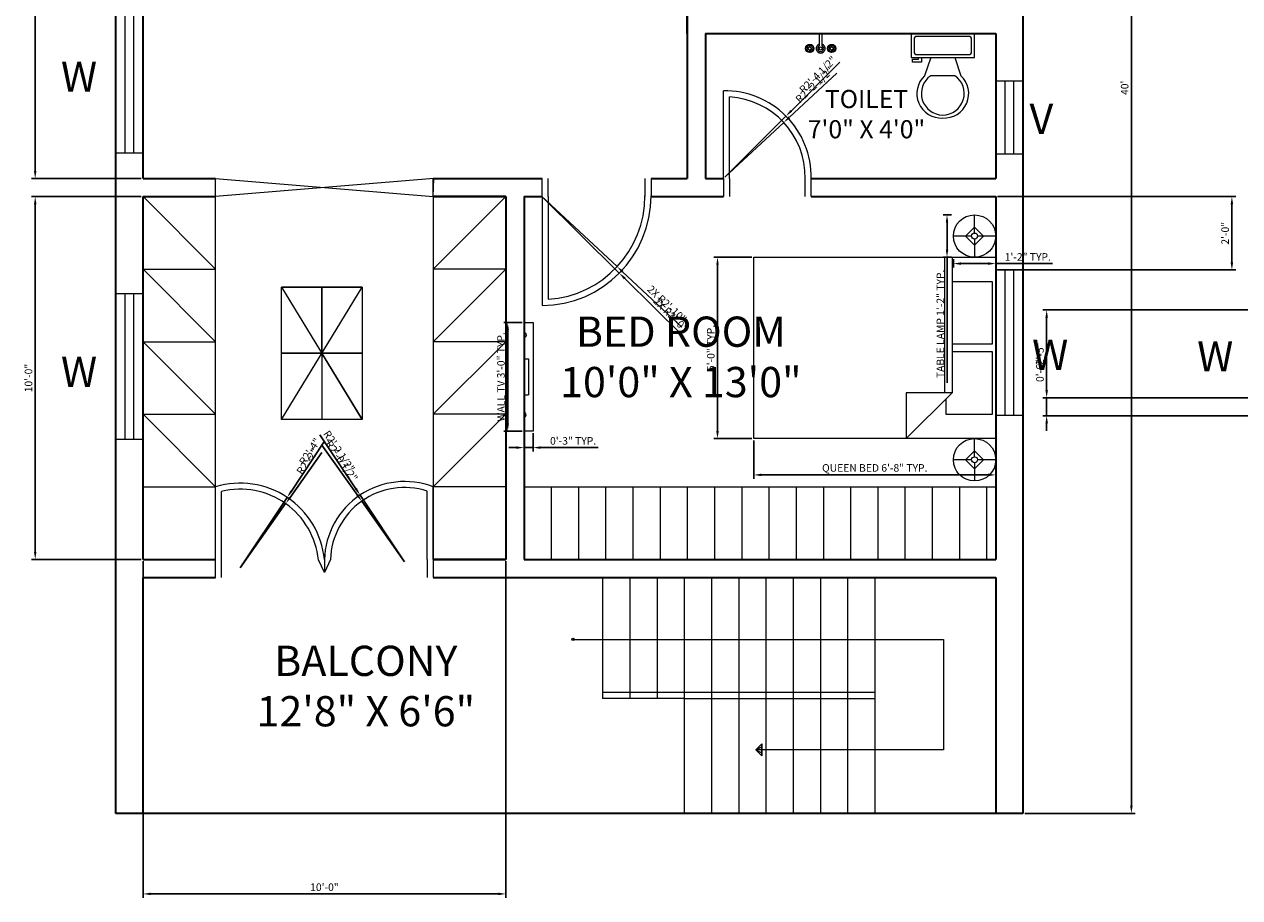
# Model space of a CAD drawing. Units: inches. Extents: x 2318 to 3542, y 1525 to 2117.
# Tile 3 of 6: x 2767 to 3169, y 1527 to 1816. Entities that reach past the tile are written whole.
import ezdxf

# ---------------------------------------------------------------- set-up
doc = ezdxf.new("R2010")
doc.units = ezdxf.units.IN
for name, color, linetype, lineweight in [('A-ANNO-DIMS', 2, 'Continuous', 18), ('A-ANNO-SYMB', 2, 'Continuous', 13), ('A-ANNO-TEXT', 7, 'Continuous', 18), ('A-AREA-IDEN', 7, 'Continuous', 25), ('A-DOOR', 4, 'Continuous', 18), ('A-EQPM', 9, 'Continuous', 18), ('A-FLOR-CASE', 8, 'Continuous', 18), ('A-FLOR-FIXT', 9, 'Continuous', 18), ('A-FLOR-STRS', 3, 'Continuous', 18), ('A-FURN', 8, 'Continuous', 18), ('A-GLAZ', 4, 'Continuous', 18), ('A-WALL', 7, 'Continuous', 35)]:
    doc.layers.add(name, color=color, linetype=linetype, lineweight=lineweight)
doc.styles.add('Annotative', font='arial.ttf')
doc.styles.get("Standard").update_dxf_attribs({"font": 'arial.ttf'})
doc.dimstyles.new('ISO-25', dxfattribs={"dimtxt": 2.5, "dimasz": 2.5, "dimexe": 1.25, "dimexo": 0.625, "dimtad": 1, "dimdec": 0, "dimlunit": 3, "dimtxsty": 'Standard', "dimcen": 2.5, "dimadec": 0, "dimazin": 0, "dimtfac": 1, "dimtdec": 0, "dimtmove": 0, "dimatfit": 3, "dimfxl": 1, "dimarcsym": 0})

# ---------------------------------------------------------------- blocks, each defined once
blk = doc.blocks.new('*D18')
at = {"layer": 'A-ANNO-DIMS', "color": 0, "lineweight": -2, "transparency": 16777216}
for p, q in [((3098.03, 2034.59), (3134.53, 2034.59)), ((3133.28, 2032.09), (3133.28, 1557.09)), ((3098.03, 1554.59), (3134.53, 1554.59))]:
    blk.add_line(p, q, dxfattribs=at)
at = {"layer": 'A-ANNO-DIMS', "color": 0, "transparency": 16777216}
for points in [[(3132.86, 2032.09), (3133.69, 2032.09), (3133.28, 2034.59)], [(3132.86, 1557.09), (3133.69, 1557.09), (3133.28, 1554.59)]]:
    blk.add_solid(points, dxfattribs=at)
at = {"layer": 'Defpoints', "color": 0, "transparency": 16777216}
for p in [(3097.41, 2034.59), (3097.41, 1554.59), (3133.28, 1554.59)]:
    blk.add_point(p, dxfattribs=at)
at = {"layer": 'A-ANNO-DIMS', "color": 0, "transparency": 16777216, "insert": (3131.38, 1794.59), "char_height": 2.5, "attachment_point": 5, "rotation": 90}
blk.add_mtext("40'", dxfattribs=at)
blk = doc.blocks.new('Bed - Queen')
for p, q in [((0, -80.00003), (0, 0)), ((0, 0), (59.99999, 0)), ((59.99999, 0), (59.99999, -80.00003)), ((7.99999, -1.2), (28.79998, -1.2)), ((7.99999, -14.4), (7.99999, -1.2)), ((28.79998, -1.2), (28.79998, -14.4)), ((31.19999, -1.2), (51.99999, -1.2)), ((31.19999, -14.4), (31.19999, -1.2)), ((51.99999, -1.2), (51.99999, -16.4)), ((0, -14.4), (44.8, -14.4)), ((59.99999, -29.6), (44.8, -14.4)), ((44.8, -14.4), (44.8, -29.6)), ((44.8, -16.8), (0, -16.8)), ((51.99999, -16.4), (46.79936, -16.4)), ((44.8, -29.6), (59.99999, -29.6)), ((59.99999, -80.00003), (0, -80.00003))]:
    blk.add_line(p, q)
blk = doc.blocks.new('Lamp - Table')
for p, q in [((0, 7), (0, 1)), ((-1, 0), (-7, 0)), ((0, 3), (-3, 0)), ((-3, 0), (0, -3)), ((3, 0), (0, 3)), ((0, -3), (3, 0)), ((1, 0), (7, 0)), ((0, -1), (0, -7))]:
    blk.add_line(p, q)
for radius in [7, 1]:
    blk.add_circle((0, 0), radius)
blk = doc.blocks.new('*U14')
for p, q in [((241.3, -152.4), (241.3, -50.8)), ((-203.2, -215.9), (-203.2, -203.2)), ((-177.8, -203.2), (-177.8, -241.3)), ((-101.6, -203.2), (-152.4, -355.6)), ((101.6, -203.2), (152.4, -355.6)), ((-254, -215.9), (-203.2, -215.9)), ((-254, -241.3), (-254, -215.9)), ((-177.8, -241.3), (-254, -241.3)), ((101.6, -355.6), (-101.6, -355.6))]:
    blk.add_line(p, q)
blk.add_lwpolyline([(266.7, -203.2), (266.7, 0), (-266.7, 0), (-266.7, -203.2)], close=True)
for points in [[(-241.3, -50.8), (-241.3, -152.4)], [(215.9, -25.4), (-215.9, -25.4)], [(-215.9, -177.8), (215.9, -177.8)]]:
    blk.add_lwpolyline(points)
for centre, radius, start, end in [((-219.075, -47.625), 22.45064, 81.8699, 188.1301), ((219.075, -47.625), 22.45064, 351.8699, 98.1301), ((-219.075, -155.575), 22.45064, 171.869898, 278.1301), ((219.075, -155.575), 22.45064, 261.8699, 8.1301), ((-12.12088, -505.93752), 205.61935, 133.01722, 273.38), ((0.94996, -504.77674), 181.02486, 124.50543, 269.7), ((-0.94742, -504.77674), 181.02486, 270.3, 55.4946), ((12.12342, -505.93752), 205.61935, 266.62, 46.9828)]:
    blk.add_arc(centre, radius, start, end)
blk = doc.blocks.new('Faucet - Bathroom top')
for p, q in [((-4.107, 0.125), (-4.375, 0.125)), ((-3.75, 0.4788), (-3.75, 0.75)), ((-3.5, 0.482), (-3.5, 0.75)), ((-3.1461, 0.125), (-2.875, 0.125)), ((3.143, 0.125), (2.875, 0.125)), ((3.5, 0.4788), (3.5, 0.75)), ((3.75, 0.482), (3.75, 0.75)), ((4.1039, 0.125), (4.375, 0.125)), ((-4.1039, -0.125), (-4.375, -0.125)), ((-3.75, -0.4821), (-3.75, -0.75)), ((-3.5, -0.4789), (-3.5, -0.75)), ((-3.143, -0.125), (-2.875, -0.125)), ((-0.5, -0.8639), (-0.5, -4.5)), ((0.5, -4.5), (0.5, -0.8631)), ((3.1461, -0.125), (2.875, -0.125)), ((3.5, -0.4821), (3.5, -0.75)), ((3.75, -0.4789), (3.75, -0.75)), ((4.107, -0.125), (4.375, -0.125))]:
    blk.add_line(p, q)
for centre, radius in [((-3.625, 0), 1.375), ((-4.625, 0), 0.2795), ((-3.625, 0), 0.5), ((-3.625, 1), 0.2795), ((-2.625, 0), 0.2795), ((0, 0), 0.5), ((3.625, 0), 1.375), ((2.625, 0), 0.2795), ((3.625, 0), 0.5), ((3.625, 1), 0.2795), ((4.625, 0), 0.2795), ((-3.625, -1), 0.2795), ((3.625, -1), 0.2795)]:
    blk.add_circle(centre, radius)
for centre, radius, start, end in [((-3.625, 0), 1, 105.2407, 164.2093), ((-3.625, 0), 1, 16.44125, 74.07887), ((0, 0), 1.5, 289.6514, 250.3603), ((0, 0), 1, 300.3431, 239.7554), ((3.625, 0), 1, 106.12, 164.0884), ((3.625, 0), 1, 16.23422, 73.90469), ((-3.625, 0), 1, 196.2342, 253.9047), ((-3.625, 0), 1, 286.12, 344.0884), ((3.625, 0), 1, 196.4413, 254.0789), ((3.625, 0), 1, 285.2407, 344.2093), ((0, -4.5), 0.5, 180, 0)]:
    blk.add_arc(centre, radius, start, end)
blk = doc.blocks.new('WIN-48x9')
for p, q in [((48, 9), (0, 9)), ((0, 9), (0, 0)), ((48, 0), (48, 9)), ((48, 6), (0, 6)), ((0, 3), (48, 3)), ((0, 0), (48, 0))]:
    blk.add_line(p, q)
blk = doc.blocks.new('VENT-24x9')
for p, q in [((0, 24), (0, 0)), ((9, 24), (0, 24)), ((3, 24), (3, 0)), ((6, 0), (6, 24)), ((9, 0), (9, 24)), ((0, 0), (9, 0))]:
    blk.add_line(p, q)
blk = doc.blocks.new('TV-36-WALL')
for p, q in [((0, 0), (0, 3)), ((0, 3), (36, 3)), ((0, 0), (0, 0)), ((0, 0), (24, 0)), ((0, 0), (12, 0)), ((12, 0), (12, 1.44)), ((12, 1.44), (23.97, 1.44)), ((23.97, 1.44), (24, 0)), ((24, 0), (23.97, 1.44)), ((36, 0), (24, 0)), ((36, 3), (36, 0))]:
    blk.add_line(p, q)
for centre, radius in [((4.16, 0), 0.848), ((30.54, 0), 0.733)]:
    blk.add_arc(centre, radius, 360, 180)
blk = doc.blocks.new('*D30')
at = {"layer": 'A-ANNO-DIMS', "color": 0, "lineweight": -2, "transparency": 16777216}
for p, q in [((3073.78, 1752.54), (3071.06, 1752.54)), ((3072.31, 1750.04), (3072.31, 1741.04)), ((3073.78, 1738.54), (3071.06, 1738.54)), ((3072.31, 1738.54), (3072.31, 1696.97))]:
    blk.add_line(p, q, dxfattribs=at)
at = {"layer": 'A-ANNO-DIMS', "color": 0, "transparency": 16777216}
for points in [[(3071.89, 1750.04), (3072.72, 1750.04), (3072.31, 1752.54)], [(3071.89, 1741.04), (3072.72, 1741.04), (3072.31, 1738.54)]]:
    blk.add_solid(points, dxfattribs=at)
at = {"layer": 'Defpoints', "color": 0, "transparency": 16777216}
for p in [(3074.41, 1752.54), (3072.31, 1738.54), (3074.41, 1738.54)]:
    blk.add_point(p, dxfattribs=at)
at = {"layer": 'A-ANNO-DIMS', "color": 0, "transparency": 16777216, "insert": (3070.43, 1716.5), "char_height": 2.5, "attachment_point": 5, "rotation": 90}
blk.add_mtext('TABLE LAMP 1\'-2" TYP.', dxfattribs=at)
blk = doc.blocks.new('*D31')
at = {"layer": 'A-ANNO-DIMS', "color": 0, "lineweight": -2, "transparency": 16777216}
for p, q in [((3074.41, 1737.91), (3074.41, 1735.19)), ((3076.91, 1736.44), (3085.91, 1736.44)), ((3088.41, 1737.91), (3088.41, 1735.19)), ((3088.41, 1736.44), (3107.16, 1736.44))]:
    blk.add_line(p, q, dxfattribs=at)
at = {"layer": 'A-ANNO-DIMS', "color": 0, "transparency": 16777216}
for points in [[(3076.91, 1736.86), (3076.91, 1736.02), (3074.41, 1736.44)], [(3085.91, 1736.86), (3085.91, 1736.02), (3088.41, 1736.44)]]:
    blk.add_solid(points, dxfattribs=at)
at = {"layer": 'Defpoints', "color": 0, "transparency": 16777216}
for p in [(3074.41, 1738.54), (3088.41, 1738.54), (3088.41, 1736.44)]:
    blk.add_point(p, dxfattribs=at)
at = {"layer": 'A-ANNO-DIMS', "color": 0, "transparency": 16777216, "insert": (3099.03, 1738.32), "char_height": 2.5, "attachment_point": 5}
blk.add_mtext('1\'-2" TYP.', dxfattribs=at)
blk = doc.blocks.new('*D36')
at = {"layer": 'A-ANNO-DIMS', "color": 0, "lineweight": -2, "transparency": 16777216}
for p, q in [((3008.41, 1677.91), (3008.41, 1665.29)), ((3088.41, 1677.91), (3088.41, 1665.29)), ((3010.91, 1666.54), (3085.91, 1666.54))]:
    blk.add_line(p, q, dxfattribs=at)
at = {"layer": 'A-ANNO-DIMS', "color": 0, "transparency": 16777216}
for points in [[(3010.91, 1666.96), (3010.91, 1666.12), (3008.41, 1666.54)], [(3085.91, 1666.96), (3085.91, 1666.12), (3088.41, 1666.54)]]:
    blk.add_solid(points, dxfattribs=at)
at = {"layer": 'Defpoints', "color": 0, "transparency": 16777216}
for p in [(3008.41, 1678.54), (3088.41, 1678.54), (3088.41, 1666.54)]:
    blk.add_point(p, dxfattribs=at)
at = {"layer": 'A-ANNO-DIMS', "color": 0, "transparency": 16777216, "insert": (3048.41, 1668.53), "char_height": 2.5, "attachment_point": 5}
blk.add_mtext('QUEEN BED 6\'-8" TYP.', dxfattribs=at)
blk = doc.blocks.new('*D37')
at = {"layer": 'A-ANNO-DIMS', "color": 0, "lineweight": -2, "transparency": 16777216}
for p, q in [((3007.78, 1738.54), (2995.16, 1738.54)), ((2996.41, 1736.04), (2996.41, 1681.04)), ((3007.78, 1678.54), (2995.16, 1678.54))]:
    blk.add_line(p, q, dxfattribs=at)
at = {"layer": 'A-ANNO-DIMS', "color": 0, "transparency": 16777216}
for points in [[(2995.99, 1736.04), (2996.82, 1736.04), (2996.41, 1738.54)], [(2995.99, 1681.04), (2996.82, 1681.04), (2996.41, 1678.54)]]:
    blk.add_solid(points, dxfattribs=at)
at = {"layer": 'Defpoints', "color": 0, "transparency": 16777216}
for p in [(3008.41, 1738.54), (2996.41, 1678.54), (3008.41, 1678.54)]:
    blk.add_point(p, dxfattribs=at)
at = {"layer": 'A-ANNO-DIMS', "color": 0, "transparency": 16777216, "insert": (2994.51, 1708.54), "char_height": 2.5, "attachment_point": 5, "rotation": 90}
blk.add_mtext('5\'-0" TYP.', dxfattribs=at)
blk = doc.blocks.new('*D40')
at = {"layer": 'A-ANNO-DIMS', "color": 0, "lineweight": -2, "transparency": 16777216}
for p, q in [((2931.78, 1716.97), (2925.76, 1716.97)), ((2927.01, 1714.47), (2927.01, 1683.47)), ((2931.78, 1680.97), (2925.76, 1680.97))]:
    blk.add_line(p, q, dxfattribs=at)
at = {"layer": 'A-ANNO-DIMS', "color": 0, "transparency": 16777216}
for points in [[(2926.59, 1714.47), (2927.42, 1714.47), (2927.01, 1716.97)], [(2926.59, 1683.47), (2927.42, 1683.47), (2927.01, 1680.97)]]:
    blk.add_solid(points, dxfattribs=at)
at = {"layer": 'Defpoints', "color": 0, "transparency": 16777216}
for p in [(2932.41, 1716.97), (2927.01, 1680.97), (2932.41, 1680.97)]:
    blk.add_point(p, dxfattribs=at)
at = {"layer": 'A-ANNO-DIMS', "color": 0, "transparency": 16777216, "insert": (2925.11, 1698.97), "char_height": 2.5, "attachment_point": 5, "rotation": 90}
blk.add_mtext('WALL TV 3\'-0" TYP.', dxfattribs=at)
blk = doc.blocks.new('*D41')
at = {"layer": 'A-ANNO-DIMS', "color": 0, "lineweight": -2, "transparency": 16777216}
for p, q in [((2932.41, 1680.35), (2932.41, 1674.32)), ((2935.41, 1680.35), (2935.41, 1674.32)), ((2929.91, 1675.57), (2927.41, 1675.57)), ((2932.41, 1675.57), (2935.41, 1675.57)), ((2937.91, 1675.57), (2956.9, 1675.57))]:
    blk.add_line(p, q, dxfattribs=at)
at = {"layer": 'A-ANNO-DIMS', "color": 0, "transparency": 16777216}
for points in [[(2929.91, 1675.99), (2929.91, 1675.16), (2932.41, 1675.57)], [(2937.91, 1675.99), (2937.91, 1675.16), (2935.41, 1675.57)]]:
    blk.add_solid(points, dxfattribs=at)
at = {"layer": 'Defpoints', "color": 0, "transparency": 16777216}
for p in [(2932.41, 1680.97), (2935.41, 1680.97), (2935.41, 1675.57)]:
    blk.add_point(p, dxfattribs=at)
at = {"layer": 'A-ANNO-DIMS', "color": 0, "transparency": 16777216, "insert": (2948.65, 1677.47), "char_height": 2.5, "attachment_point": 5}
blk.add_mtext('0\'-3" TYP.', dxfattribs=at)
blk = doc.blocks.new('*D57')
at = {"layer": 'A-ANNO-DIMS', "color": 0, "lineweight": -2, "transparency": 16777216}
for p, q in [((2806.41, 1637.97), (2806.41, 1526.69)), ((2926.41, 1637.97), (2926.41, 1526.69)), ((2808.91, 1527.94), (2923.91, 1527.94))]:
    blk.add_line(p, q, dxfattribs=at)
at = {"layer": 'A-ANNO-DIMS', "color": 0, "transparency": 16777216}
for points in [[(2808.91, 1528.36), (2808.91, 1527.53), (2806.41, 1527.94)], [(2923.91, 1528.36), (2923.91, 1527.53), (2926.41, 1527.94)]]:
    blk.add_solid(points, dxfattribs=at)
at = {"layer": 'Defpoints', "color": 0, "transparency": 16777216}
for p in [(2806.41, 1638.59), (2926.41, 1638.59), (2926.41, 1527.94)]:
    blk.add_point(p, dxfattribs=at)
at = {"layer": 'A-ANNO-DIMS', "color": 0, "transparency": 16777216, "insert": (2866.41, 1529.84), "char_height": 2.5, "attachment_point": 5}
blk.add_mtext('10\'-0"', dxfattribs=at)
blk = doc.blocks.new('*D58')
at = {"layer": 'A-ANNO-DIMS', "color": 0, "lineweight": -2, "transparency": 16777216}
for p, q in [((2805.78, 1758.59), (2769.51, 1758.59)), ((2770.76, 1641.09), (2770.76, 1756.09)), ((2805.78, 1638.59), (2769.51, 1638.59))]:
    blk.add_line(p, q, dxfattribs=at)
at = {"layer": 'A-ANNO-DIMS', "color": 0, "transparency": 16777216}
for points in [[(2770.34, 1756.09), (2771.17, 1756.09), (2770.76, 1758.59)], [(2770.34, 1641.09), (2771.17, 1641.09), (2770.76, 1638.59)]]:
    blk.add_solid(points, dxfattribs=at)
at = {"layer": 'Defpoints', "color": 0, "transparency": 16777216}
for p in [(2770.76, 1758.59), (2806.41, 1758.59), (2806.41, 1638.59)]:
    blk.add_point(p, dxfattribs=at)
at = {"layer": 'A-ANNO-DIMS', "color": 0, "transparency": 16777216, "insert": (2768.86, 1698.59), "char_height": 2.5, "attachment_point": 5, "rotation": 90}
blk.add_mtext('10\'-0"', dxfattribs=at)
blk = doc.blocks.new('*D63')
at = {"layer": 'A-ANNO-DIMS', "color": 0, "lineweight": -2, "transparency": 16777216}
for p, q in [((2805.78, 1899.59), (2769.51, 1899.59)), ((2770.76, 1767.09), (2770.76, 1897.09)), ((2805.78, 1764.59), (2769.51, 1764.59))]:
    blk.add_line(p, q, dxfattribs=at)
at = {"layer": 'A-ANNO-DIMS', "color": 0, "transparency": 16777216}
for points in [[(2770.34, 1897.09), (2771.17, 1897.09), (2770.76, 1899.59)], [(2770.34, 1767.09), (2771.17, 1767.09), (2770.76, 1764.59)]]:
    blk.add_solid(points, dxfattribs=at)
at = {"layer": 'Defpoints', "color": 0, "transparency": 16777216}
for p in [(2770.76, 1899.59), (2806.41, 1899.59), (2806.41, 1764.59)]:
    blk.add_point(p, dxfattribs=at)
at = {"layer": 'A-ANNO-DIMS', "color": 0, "transparency": 16777216, "insert": (2768.86, 1832.09), "char_height": 2.5, "attachment_point": 5, "rotation": 90}
blk.add_mtext('11\'-3"', dxfattribs=at)
blk = doc.blocks.new('*D64')
at = {"layer": 'A-ANNO-DIMS', "color": 0, "lineweight": -2, "transparency": 16777216}
for p, q in [((3394.81, 1721.09), (3104.01, 1721.09)), ((3105.26, 1694.59), (3105.26, 1718.59)), ((3394.81, 1692.09), (3104.01, 1692.09))]:
    blk.add_line(p, q, dxfattribs=at)
at = {"layer": 'A-ANNO-DIMS', "color": 0, "transparency": 16777216}
for points in [[(3104.85, 1718.59), (3105.68, 1718.59), (3105.26, 1721.09)], [(3104.85, 1694.59), (3105.68, 1694.59), (3105.26, 1692.09)]]:
    blk.add_solid(points, dxfattribs=at)
at = {"layer": 'Defpoints', "color": 0, "transparency": 16777216}
for p in [(3105.26, 1721.09), (3395.43, 1721.09), (3395.43, 1692.09)]:
    blk.add_point(p, dxfattribs=at)
at = {"layer": 'A-ANNO-DIMS', "color": 0, "transparency": 16777216, "insert": (3103.36, 1706.59), "char_height": 2.5, "attachment_point": 5, "rotation": 90}
blk.add_mtext('2\'-5"', dxfattribs=at)
blk = doc.blocks.new('*D65')
at = {"layer": 'A-ANNO-DIMS', "color": 0, "lineweight": -2, "transparency": 16777216}
for p, q in [((3105.26, 1694.59), (3105.26, 1704.98)), ((3400.81, 1692.09), (3104.01, 1692.09)), ((3105.26, 1686.09), (3105.26, 1692.09)), ((3400.81, 1686.09), (3104.01, 1686.09)), ((3105.26, 1683.59), (3105.26, 1681.09))]:
    blk.add_line(p, q, dxfattribs=at)
at = {"layer": 'A-ANNO-DIMS', "color": 0, "transparency": 16777216}
for points in [[(3104.85, 1694.59), (3105.68, 1694.59), (3105.26, 1692.09)], [(3104.85, 1683.59), (3105.68, 1683.59), (3105.26, 1686.09)]]:
    blk.add_solid(points, dxfattribs=at)
at = {"layer": 'Defpoints', "color": 0, "transparency": 16777216}
for p in [(3105.26, 1692.09), (3401.43, 1692.09), (3401.43, 1686.09)]:
    blk.add_point(p, dxfattribs=at)
at = {"layer": 'A-ANNO-DIMS', "color": 0, "transparency": 16777216, "insert": (3103.36, 1701.04), "char_height": 2.5, "attachment_point": 5, "rotation": 90}
blk.add_mtext('0\'-6"', dxfattribs=at)
blk = doc.blocks.new('*D73')
at = {"layer": 'A-ANNO-DIMS', "color": 0, "lineweight": -2, "transparency": 16777216}
for p, q in [((3089.03, 1758.59), (3167.77, 1758.59)), ((3166.52, 1736.85), (3166.52, 1756.09)), ((3089.03, 1734.35), (3167.77, 1734.35))]:
    blk.add_line(p, q, dxfattribs=at)
at = {"layer": 'A-ANNO-DIMS', "color": 0, "transparency": 16777216}
for points in [[(3166.1, 1756.09), (3166.93, 1756.09), (3166.52, 1758.59)], [(3166.1, 1736.85), (3166.93, 1736.85), (3166.52, 1734.35)]]:
    blk.add_solid(points, dxfattribs=at)
at = {"layer": 'Defpoints', "color": 0, "transparency": 16777216}
for p in [(3088.41, 1758.59), (3166.52, 1758.59), (3088.41, 1734.35)]:
    blk.add_point(p, dxfattribs=at)
at = {"layer": 'A-ANNO-DIMS', "color": 0, "transparency": 16777216, "insert": (3164.61, 1746.47), "char_height": 2.5, "attachment_point": 5, "rotation": 90}
blk.add_mtext('2\'-0"', dxfattribs=at)
blk = doc.blocks.new('*D81')
at = {"layer": 'A-ANNO-DIMS', "color": 0, "lineweight": -2, "transparency": 16777216}
for p, q in [((2938.25, 1758.75), (2963.93, 1733.3)), ((2984.91, 1712.49), (2965.7, 1731.54))]:
    blk.add_line(p, q, dxfattribs=at)
at = {"layer": 'A-ANNO-DIMS', "color": 0, "transparency": 16777216}
blk.add_solid([(2966, 1731.83), (2965.41, 1731.24), (2963.93, 1733.3)], dxfattribs=at)
at = {"layer": 'Defpoints', "color": 0, "transparency": 16777216}
for p in [(2938.25, 1758.75), (2963.93, 1733.3)]:
    blk.add_point(p, dxfattribs=at)
at = {"layer": 'A-ANNO-DIMS', "color": 0, "transparency": 16777216, "insert": (2980.68, 1719.37), "char_height": 2.5, "attachment_point": 5, "rotation": 315.2514}
blk.add_mtext('2X R3\'-0"', dxfattribs=at)
blk = doc.blocks.new('*D84')
at = {"layer": 'A-ANNO-DIMS', "color": 0, "lineweight": -2, "transparency": 16777216}
for p, q in [((3036.86, 1803.04), (3020.82, 1787.01)), ((2998.88, 1765.06), (3019.05, 1785.24))]:
    blk.add_line(p, q, dxfattribs=at)
at = {"layer": 'A-ANNO-DIMS', "color": 0, "transparency": 16777216}
blk.add_solid([(3020.53, 1787.3), (3021.12, 1786.71), (3019.05, 1785.24)], dxfattribs=at)
at = {"layer": 'Defpoints', "color": 0, "transparency": 16777216}
for p in [(3019.05, 1785.24), (2998.88, 1765.06)]:
    blk.add_point(p, dxfattribs=at)
at = {"layer": 'A-ANNO-DIMS', "color": 0, "transparency": 16777216, "insert": (3029.8, 1798.7), "char_height": 2.5, "attachment_point": 5, "rotation": 45}
blk.add_mtext('R2\'-4 1/2"', dxfattribs=at)
blk = doc.blocks.new('*D90')
at = {"layer": 'A-ANNO-DIMS', "color": 0, "lineweight": -2, "transparency": 16777216}
for p, q in [((2866.25, 1677.36), (2855.47, 1661.19)), ((2838.57, 1635.84), (2854.09, 1659.11))]:
    blk.add_line(p, q, dxfattribs=at)
at = {"layer": 'A-ANNO-DIMS', "color": 0, "transparency": 16777216}
blk.add_solid([(2855.13, 1661.42), (2855.82, 1660.96), (2854.09, 1659.11)], dxfattribs=at)
at = {"layer": 'Defpoints', "color": 0, "transparency": 16777216}
for p in [(2854.09, 1659.11), (2838.57, 1635.84)]:
    blk.add_point(p, dxfattribs=at)
at = {"layer": 'A-ANNO-DIMS', "color": 0, "transparency": 16777216, "insert": (2861.83, 1674.12), "char_height": 2.5, "attachment_point": 5, "rotation": 56.3095}
blk.add_mtext('R2\'-4"', dxfattribs=at)
blk = doc.blocks.new('*D91')
at = {"layer": 'A-ANNO-DIMS', "color": 0, "lineweight": -2, "transparency": 16777216}
for p, q in [((2864.91, 1679.84), (2876.82, 1661.97)), ((2892.92, 1637.83), (2878.21, 1659.89))]:
    blk.add_line(p, q, dxfattribs=at)
at = {"layer": 'A-ANNO-DIMS', "color": 0, "transparency": 16777216}
blk.add_solid([(2877.17, 1662.21), (2876.47, 1661.74), (2878.21, 1659.89)], dxfattribs=at)
at = {"layer": 'Defpoints', "color": 0, "transparency": 16777216}
for p in [(2878.21, 1659.89), (2892.92, 1637.83)]:
    blk.add_point(p, dxfattribs=at)
at = {"layer": 'A-ANNO-DIMS', "color": 0, "transparency": 16777216, "insert": (2870.98, 1674.2), "char_height": 2.5, "attachment_point": 5, "rotation": 303.6886}
blk.add_mtext('R2\'-2 1/2"', dxfattribs=at)
blk = doc.blocks.new('*D101')
at = {"layer": 'A-ANNO-DIMS', "color": 0, "lineweight": -2, "transparency": 16777216}
for p, q in [((3035.89, 1799.43), (3020.16, 1784.82)), ((2998.88, 1765.06), (3018.32, 1783.12))]:
    blk.add_line(p, q, dxfattribs=at)
at = {"layer": 'A-ANNO-DIMS', "color": 0, "transparency": 16777216}
blk.add_solid([(3019.87, 1785.12), (3020.44, 1784.51), (3018.32, 1783.12)], dxfattribs=at)
at = {"layer": 'Defpoints', "color": 0, "transparency": 16777216}
for p in [(3018.32, 1783.12), (2998.88, 1765.06)]:
    blk.add_point(p, dxfattribs=at)
at = {"layer": 'A-ANNO-DIMS', "color": 0, "transparency": 16777216, "insert": (3028.69, 1795.35), "char_height": 2.5, "attachment_point": 5, "rotation": 42.874}
blk.add_mtext('R2\'-2 1/2"', dxfattribs=at)
blk = doc.blocks.new('*D104')
at = {"layer": 'A-ANNO-DIMS', "color": 0, "lineweight": -2, "transparency": 16777216}
for p, q in [((2865.6, 1676.43), (2877.31, 1659.88)), ((2892.92, 1637.83), (2878.75, 1657.84))]:
    blk.add_line(p, q, dxfattribs=at)
at = {"layer": 'A-ANNO-DIMS', "color": 0, "transparency": 16777216}
blk.add_solid([(2877.65, 1660.13), (2876.97, 1659.64), (2878.75, 1657.84)], dxfattribs=at)
at = {"layer": 'Defpoints', "color": 0, "transparency": 16777216}
for p in [(2878.75, 1657.84), (2892.92, 1637.83)]:
    blk.add_point(p, dxfattribs=at)
at = {"layer": 'A-ANNO-DIMS', "color": 0, "transparency": 16777216, "insert": (2871.82, 1670.96), "char_height": 2.5, "attachment_point": 5, "rotation": 305.2803}
blk.add_mtext('R2\'-0 1/2"', dxfattribs=at)
blk = doc.blocks.new('*D108')
at = {"layer": 'A-ANNO-DIMS', "color": 0, "lineweight": -2, "transparency": 16777216}
for p, q in [((2938.25, 1758.75), (2963.21, 1735.43)), ((2984.63, 1715.41), (2965.03, 1733.72))]:
    blk.add_line(p, q, dxfattribs=at)
at = {"layer": 'A-ANNO-DIMS', "color": 0, "transparency": 16777216}
blk.add_solid([(2965.32, 1734.03), (2964.75, 1733.42), (2963.21, 1735.43)], dxfattribs=at)
at = {"layer": 'Defpoints', "color": 0, "transparency": 16777216}
for p in [(2938.25, 1758.75), (2963.21, 1735.43)]:
    blk.add_point(p, dxfattribs=at)
at = {"layer": 'A-ANNO-DIMS', "color": 0, "transparency": 16777216, "insert": (2979.48, 1722.82), "char_height": 2.5, "attachment_point": 5, "rotation": 316.9388}
blk.add_mtext('2X R2\'-10"', dxfattribs=at)
blk = doc.blocks.new('*D110')
at = {"layer": 'A-ANNO-DIMS', "color": 0, "lineweight": -2, "transparency": 16777216}
for p, q in [((2865.56, 1673.95), (2855.03, 1659.07)), ((2838.57, 1635.84), (2853.58, 1657.03))]:
    blk.add_line(p, q, dxfattribs=at)
at = {"layer": 'A-ANNO-DIMS', "color": 0, "transparency": 16777216}
blk.add_solid([(2854.69, 1659.31), (2855.37, 1658.83), (2853.58, 1657.03)], dxfattribs=at)
at = {"layer": 'Defpoints', "color": 0, "transparency": 16777216}
for p in [(2853.58, 1657.03), (2838.57, 1635.84)]:
    blk.add_point(p, dxfattribs=at)
at = {"layer": 'A-ANNO-DIMS', "color": 0, "transparency": 16777216, "insert": (2861.06, 1670.84), "char_height": 2.5, "attachment_point": 5, "rotation": 54.689}
blk.add_mtext('R2\'-2"', dxfattribs=at)

msp = doc.modelspace()

# ---------------------------------------------------------------- linework, layer by layer
at = {"layer": 'A-ANNO-SYMB'}
for p, q in [((2866.41, 1634.31), (2864.42, 1638.4)), ((2866.41, 1638.59), (2866.41, 1634.31)), ((2868.41, 1638.53), (2866.41, 1634.31)), ((2948.61, 1612.14), (3071.19, 1612.14)), ((3071.19, 1612.14), (3071.19, 1575.58)), ((3009.08, 1575.58), (3011.08, 1577.58)), ((3009.08, 1575.58), (3011.08, 1576.58)), ((3011.08, 1576.58), (3009.08, 1575.58)), ((3011.08, 1575.58), (3011.08, 1577.58)), ((3011.08, 1577.58), (3011.08, 1575.58)), ((3011.08, 1577.58), (3011.08, 1573.58)), ((3011.08, 1575.58), (3009.08, 1575.58)), ((3011.08, 1573.58), (3009.08, 1575.58)), ((3009.08, 1575.58), (3011.08, 1574.58)), ((3071.19, 1575.58), (3011.08, 1575.58)), ((3011.08, 1575.58), (3011.08, 1573.58)), ((3011.08, 1573.58), (3011.08, 1575.58))]:
    msp.add_line(p, q, dxfattribs=at)
msp.add_circle((2948.61, 1612.14), 0.399, dxfattribs=at)
at = {"layer": 'A-DOOR'}
for p, q in [((2998.41, 1764.59), (2998.41, 1793.59)), ((3000.41, 1793.56), (3000.41, 1793.59)), ((3000.41, 1764.59), (3000.41, 1791.55)), ((2830.41, 1758.59), (2830.41, 1764.59)), ((2902.41, 1758.59), (2902.41, 1764.59)), ((2938.41, 1758.59), (2938.41, 1764.59)), ((2940.41, 1758.59), (2940.41, 1764.59)), ((2972.41, 1764.59), (2972.41, 1758.59)), ((2974.41, 1764.59), (2974.41, 1758.59)), ((2998.41, 1764.59), (2998.41, 1758.59)), ((3000.41, 1764.59), (3000.41, 1758.59)), ((3025.41, 1758.59), (3025.41, 1764.59)), ((3027.41, 1758.59), (3027.41, 1764.59)), ((2938.41, 1758.59), (2938.41, 1722.59)), ((2940.41, 1758.59), (2940.41, 1724.66)), ((2830.41, 1662.59), (2830.41, 1662.59)), ((2832.41, 1638.59), (2832.41, 1661.07)), ((2900.41, 1638.59), (2900.41, 1661.18)), ((2902.41, 1638.59), (2902.41, 1662.59)), ((2830.41, 1632.59), (2830.41, 1638.59)), ((2832.41, 1632.59), (2832.41, 1638.59)), ((2900.41, 1638.59), (2900.41, 1632.59)), ((2902.41, 1638.59), (2902.41, 1632.59))]:
    msp.add_line(p, q, dxfattribs=at)
msp.add_lwpolyline([(2830.41, 1764.59), (2902.41, 1758.59), (2902.56, 1764.59), (2830.41, 1758.59), (2830.41, 1758.59)], dxfattribs=at)
for centre, radius, start, end in [((2998.88, 1765.06), 28.53, 359.0538, 90.9462), ((2998.88, 1765.06), 26.53, 359.0538, 86.6967), ((2938.25, 1758.75), 36.16, 170.7039, 172.393), ((2938.25, 1758.75), 36.16, 270.2518, 0.2518), ((2938.25, 1758.75), 34.16, 273.6236, 0.2518), ((2938.25, 1758.75), 34.16, 270.2518, 270.2666), ((2892.92, 1637.83), 26.52, 69.0362, 178.344), ((2838.57, 1635.84), 27.97, 5.6467, 106.9732), ((2838.57, 1635.84), 25.97, 5.6467, 103.7328), ((2892.92, 1637.83), 24.52, 72.2178, 178.344)]:
    msp.add_arc(centre, radius, start, end, dxfattribs=at)
at = {"layer": 'A-FLOR-CASE'}
for p, q in [((2932.41, 1662.59), (3088.41, 1662.59)), ((2941.41, 1662.59), (2941.41, 1638.59)), ((2950.41, 1662.59), (2950.41, 1638.59)), ((2959.41, 1662.59), (2959.41, 1638.59)), ((2968.41, 1662.59), (2968.41, 1638.59)), ((2977.41, 1662.59), (2977.41, 1638.59)), ((2986.41, 1662.59), (2986.41, 1638.59)), ((2995.41, 1662.59), (2995.41, 1638.59)), ((3004.41, 1662.59), (3004.41, 1638.59)), ((3013.41, 1662.59), (3013.41, 1638.59)), ((3022.41, 1662.59), (3022.41, 1638.59)), ((3031.41, 1662.59), (3031.41, 1638.59)), ((3040.41, 1662.59), (3040.41, 1638.59)), ((3049.41, 1662.59), (3049.41, 1638.59)), ((3058.41, 1662.59), (3058.41, 1638.59)), ((3067.41, 1662.59), (3067.41, 1638.59)), ((3076.41, 1662.59), (3076.41, 1638.59)), ((3085.41, 1662.59), (3085.41, 1638.59))]:
    msp.add_line(p, q, dxfattribs=at)
at = {"layer": 'A-FLOR-STRS'}
for p, q in [((2958.41, 1632.59), (2958.41, 1592.59)), ((2967.41, 1632.59), (2967.41, 1592.59)), ((2976.41, 1632.59), (2976.41, 1592.59)), ((2985.41, 1632.59), (2985.41, 1554.59)), ((2994.41, 1632.59), (2994.41, 1554.59)), ((3003.41, 1632.59), (3003.41, 1554.59)), ((3012.41, 1632.59), (3012.41, 1554.59)), ((3021.41, 1632.59), (3021.41, 1554.59)), ((3030.41, 1632.59), (3030.41, 1554.59)), ((3039.41, 1632.59), (3039.41, 1554.59)), ((3048.41, 1632.59), (3048.41, 1554.59)), ((2985.41, 1594.59), (2958.41, 1594.59)), ((2985.41, 1592.59), (2958.41, 1592.59)), ((3048.41, 1594.59), (2985.41, 1594.59)), ((2985.41, 1594.59), (2985.41, 1554.59)), ((2985.41, 1592.59), (3048.41, 1592.59))]:
    msp.add_line(p, q, dxfattribs=at)
at = {"layer": 'A-FURN'}
for p, q in [((2830.41, 1734.59), (2806.41, 1758.59)), ((2830.41, 1638.59), (2830.41, 1758.59)), ((2902.41, 1758.59), (2902.41, 1638.59)), ((2902.41, 1734.59), (2926.41, 1758.59)), ((2806.41, 1734.59), (2830.41, 1734.59)), ((2830.41, 1710.59), (2806.41, 1734.59)), ((2926.41, 1734.59), (2902.41, 1734.59)), ((2902.41, 1710.59), (2926.41, 1734.59)), ((2926.41, 1734.59), (2902.41, 1734.59)), ((2852.19, 1684.91), (2878.92, 1728.69)), ((2878.92, 1728.69), (2852.19, 1728.69)), ((2852.19, 1728.69), (2878.92, 1684.91)), ((2865.56, 1706.8), (2865.56, 1728.69)), ((2865.56, 1728.69), (2865.56, 1684.91)), ((2806.41, 1710.59), (2830.41, 1710.59)), ((2830.41, 1686.59), (2806.41, 1710.59)), ((2926.41, 1710.59), (2902.41, 1710.59)), ((2902.41, 1686.59), (2926.41, 1710.59)), ((2878.92, 1706.8), (2852.19, 1706.8)), ((2852.19, 1706.8), (2865.56, 1706.8)), ((2878.92, 1684.91), (2865.56, 1706.8)), ((2865.56, 1706.8), (2878.92, 1706.8)), ((2806.41, 1686.59), (2830.41, 1686.59)), ((2830.41, 1662.59), (2806.41, 1686.59)), ((2926.41, 1686.59), (2902.41, 1686.59)), ((2902.41, 1662.59), (2926.41, 1686.59)), ((2806.41, 1662.59), (2830.41, 1662.59)), ((2926.41, 1662.59), (2902.41, 1662.59))]:
    msp.add_line(p, q, dxfattribs=at)
msp.add_lwpolyline([(2852.19, 1684.91), (2852.19, 1728.69), (2878.92, 1728.69), (2878.92, 1684.91)], close=True, dxfattribs=at)
at = {"layer": 'A-WALL'}
for p, q in [((2797.41, 1554.59), (2797.41, 2034.59)), ((3097.41, 2034.59), (3097.41, 1554.59)), ((2806.41, 1764.59), (2806.41, 1899.59)), ((2986.41, 1812.59), (2986.41, 1818.59)), ((2986.41, 1818.59), (2986.41, 1764.59)), ((2986.41, 1812.59), (2986.41, 1764.59)), ((2992.41, 1812.59), (2992.41, 1764.59)), ((2992.41, 1812.59), (3088.41, 1812.59)), ((3088.41, 1812.59), (3088.41, 1764.59)), ((2806.41, 1764.59), (2830.41, 1764.59)), ((2902.41, 1764.59), (2938.41, 1764.59)), ((2974.41, 1764.59), (2986.41, 1764.59)), ((2992.41, 1764.59), (2998.41, 1764.59)), ((2992.41, 1764.59), (2998.41, 1764.59)), ((3027.41, 1764.59), (3088.41, 1764.59)), ((2806.41, 1758.59), (2830.41, 1758.59)), ((2806.41, 1638.59), (2806.41, 1758.59)), ((2806.41, 1758.59), (2830.41, 1758.59)), ((2926.41, 1758.59), (2902.41, 1758.59)), ((2902.41, 1758.59), (2926.41, 1758.59)), ((2926.41, 1758.59), (2926.41, 1638.59)), ((2932.41, 1758.59), (2932.41, 1638.59)), ((2932.41, 1758.59), (2938.41, 1758.59)), ((2932.41, 1758.59), (2938.41, 1758.59)), ((2974.41, 1758.59), (2998.41, 1758.59)), ((3027.41, 1758.59), (3088.41, 1758.59)), ((3088.41, 1758.59), (3088.41, 1638.59)), ((2806.41, 1638.59), (2830.41, 1638.59)), ((2926.41, 1638.59), (2902.41, 1638.59)), ((2902.41, 1638.59), (2926.41, 1638.59)), ((2932.41, 1638.59), (3088.41, 1638.59)), ((2806.41, 1554.59), (2806.41, 1632.59)), ((2806.41, 1632.59), (2830.41, 1632.59)), ((2806.41, 1632.59), (2830.41, 1632.59)), ((2902.41, 1632.59), (3088.41, 1632.59)), ((3088.41, 1632.59), (3088.41, 1554.59)), ((3097.41, 1554.59), (2797.41, 1554.59))]:
    msp.add_line(p, q, dxfattribs=at)

# ---------------------------------------------------------------- block references
at = {"layer": 'A-EQPM', "rotation": 270.0000000000019}
msp.add_blockref('TV-36-WALL', (2932.41, 1716.97), dxfattribs=at)
at = {"layer": 'A-FLOR-FIXT', "rotation": 180}
msp.add_blockref('Faucet - Bathroom top', (3030.53, 1807.59), dxfattribs=at)
at = {"layer": 'A-FLOR-FIXT', "xscale": 0.0393700787401575, "yscale": 0.0393700787401575, "zscale": 0.0393700787401575}
msp.add_blockref('*U14', (3070.91, 1812.59), dxfattribs=at)
at = {"layer": 'A-FURN', "rotation": 270}
for name, p in [('Lamp - Table', (3081.41, 1745.54)), ('Bed - Queen', (3088.41, 1738.54)), ('Lamp - Table', (3081.41, 1671.54))]:
    msp.add_blockref(name, p, dxfattribs=at)
at = {"layer": 'A-GLAZ'}
for name, p, rotation in [('WIN-48x9', (2806.41, 1773.07), 90.00000000000179), ('VENT-24x9', (3097.41, 1796.75), 180), ('WIN-48x9', (3097.41, 1686.35), 89.99999999999969), ('WIN-48x9', (2806.41, 1678.4), 90.00000000000179)]:
    msp.add_blockref(name, p, dxfattribs=dict(at, rotation=rotation))

# ---------------------------------------------------------------- texts
at = {"layer": 'A-ANNO-TEXT', "char_height": 10, "attachment_point": 1}
for s, insert in [('\\pxt1;W', (2779.26, 1803.28)), ('\\pxt1;V', (3099.58, 1789.32)), ('\\pxt1;W', (3100.44, 1711.27)), ('\\pxt1;W', (3155.02, 1710.77)), ('\\pxt1;W', (2779.26, 1705.65))]:
    msp.add_mtext_dynamic_manual_height_columns(s, width=219.3474, gutter_width=12.5, heights=[0], dxfattribs=dict(at, insert=insert))
at = {"layer": 'A-AREA-IDEN', "insert": (3022.26, 1793.88), "char_height": 6, "attachment_point": 1}
msp.add_mtext_dynamic_manual_height_columns('\\pxqc,t2;TOILET\\P7\'0" X 4\'0"', width=46.835, gutter_width=12.5, heights=[0], dxfattribs=at)
at = {"layer": 'A-AREA-IDEN', "char_height": 10, "width": 132.7792, "attachment_point": 1, "style": 'Annotative'}
for s, insert in [('\\pxqc;BED ROOM\\P10\'0" X 13\'0"', (2917.89, 1718.92)), ('\\pxqc;BALCONY\\P12\'8" X 6\'6"', (2813.71, 1610.04))]:
    msp.add_mtext(s, dxfattribs=dict(at, insert=insert))

# ---------------------------------------------------------------- dimensions: what is measured, and where the dimension line sits
at = {"layer": 'A-ANNO-DIMS'}
for base, p1, p2, override, picture, middle in [((3133.28, 1554.59), (3097.41, 2034.59), (3097.41, 1554.59), {"dimclrd": 0, "dimclre": 0, "dimclrt": 0}, '*D18', (3131.38, 1794.59)), ((2770.76, 1899.59), (2806.41, 1764.59), (2806.41, 1899.59), {"dimdec": 1, "dimlfac": 1, "dimrnd": 0, "dimzin": 1, "dimdsep": 46, "dimlunit": 4, "dimfrac": 2}, '*D63', (2768.86, 1832.09)), ((2770.76, 1758.59), (2806.41, 1638.59), (2806.41, 1758.59), {"dimdec": 1, "dimlfac": 1, "dimrnd": 0, "dimzin": 1, "dimdsep": 46, "dimlunit": 4, "dimfrac": 2}, '*D58', (2768.86, 1698.59)), ((3166.52, 1758.59), (3088.41, 1734.35), (3088.41, 1758.59), {"dimdec": 1, "dimlfac": 1, "dimrnd": 0, "dimzin": 1, "dimdsep": 46, "dimlunit": 4, "dimfrac": 2}, '*D73', (3164.61, 1746.47)), ((3105.26, 1721.09), (3395.43, 1692.09), (3395.43, 1721.09), {"dimdec": 1, "dimlfac": 1, "dimrnd": 0, "dimzin": 1, "dimdsep": 46, "dimlunit": 4, "dimfrac": 2}, '*D64', (3103.36, 1706.59)), ((3105.26, 1692.09), (3401.43, 1686.09), (3401.43, 1692.09), {"dimdec": 1, "dimlfac": 1, "dimrnd": 0, "dimzin": 1, "dimdsep": 46, "dimlunit": 4, "dimfrac": 2}, '*D65', (3103.36, 1701.04))]:
    dim = msp.add_linear_dim(base=base, p1=p1, p2=p2, angle=90, dimstyle='ISO-25', override=override, dxfattribs=at)
    dim.commit()
    dim.dimension.update_dxf_attribs({"geometry": picture, "text_midpoint": middle})
for center, mpoint, picture, middle in [((2998.88, 1765.06), (3019.05, 1785.24), '*D84', (3031.16, 1797.34)), ((2998.88, 1765.06), (3018.32, 1783.12), '*D101', (3029.99, 1793.95)), ((2892.92, 1637.83), (2878.21, 1659.89), '*D91', (2869.38, 1673.13)), ((2838.57, 1635.84), (2854.09, 1659.11), '*D90', (2863.4, 1673.08)), ((2892.92, 1637.83), (2878.75, 1657.84), '*D104', (2870.26, 1669.86)), ((2838.57, 1635.84), (2853.58, 1657.03), '*D110', (2862.59, 1669.75))]:
    dim = msp.add_radius_dim(center=center, mpoint=mpoint, dimstyle='ISO-25', override={"dimdec": 1, "dimlfac": 1, "dimrnd": 0, "dimzin": 1, "dimdsep": 46, "dimlunit": 4, "dimfrac": 2}, dxfattribs=at)
    dim.commit()
    dim.dimension.update_dxf_attribs({"geometry": picture, "text_midpoint": middle, "dimtype": 164})
for mpoint, picture, middle in [((2963.93, 1733.3), '*D81', (2979.34, 1718.02)), ((2963.21, 1735.43), '*D108', (2978.18, 1721.43))]:
    dim = msp.add_radius_dim(center=(2938.25, 1758.75), mpoint=mpoint, text='2X <>', dimstyle='ISO-25', override={"dimdec": 1, "dimlfac": 1, "dimrnd": 0, "dimzin": 1, "dimdsep": 46, "dimlunit": 4, "dimfrac": 2}, dxfattribs=at)
    dim.commit()
    dim.dimension.update_dxf_attribs({"geometry": picture, "text_midpoint": middle, "dimtype": 164})
for base, p1, p2, text, picture, middle in [((3072.31, 1738.54), (3074.41, 1752.54), (3074.41, 1738.54), 'TABLE LAMP <> TYP.', '*D30', (3070.43, 1716.5)), ((2996.41, 1678.54), (3008.41, 1738.54), (3008.41, 1678.54), '<> TYP.', '*D37', (2994.51, 1708.54)), ((2927.01, 1680.97), (2932.41, 1716.97), (2932.41, 1680.97), 'WALL TV <> TYP.', '*D40', (2925.11, 1698.97))]:
    dim = msp.add_linear_dim(base=base, p1=p1, p2=p2, angle=270, text=text, dimstyle='ISO-25', override={"dimdec": 1, "dimlfac": 1, "dimrnd": 0, "dimzin": 1, "dimdsep": 46, "dimlunit": 4, "dimfrac": 2}, dxfattribs=at)
    dim.commit()
    dim.dimension.update_dxf_attribs({"geometry": picture, "text_midpoint": middle})
for base, p1, p2, text, picture, middle in [((3088.41, 1736.44), (3074.41, 1738.54), (3088.41, 1738.54), '<> TYP.', '*D31', (3099.03, 1738.32)), ((2935.41, 1675.57), (2932.41, 1680.97), (2935.41, 1680.97), '<> TYP.', '*D41', (2948.65, 1677.47)), ((3088.41, 1666.54), (3008.41, 1678.54), (3088.41, 1678.54), 'QUEEN BED <> TYP.', '*D36', (3048.41, 1668.53))]:
    dim = msp.add_linear_dim(base=base, p1=p1, p2=p2, text=text, dimstyle='ISO-25', override={"dimdec": 1, "dimlfac": 1, "dimrnd": 0, "dimzin": 1, "dimdsep": 46, "dimlunit": 4, "dimfrac": 2}, dxfattribs=at)
    dim.commit()
    dim.dimension.update_dxf_attribs({"geometry": picture, "text_midpoint": middle})
dim = msp.add_linear_dim(base=(2926.41, 1527.94), p1=(2806.41, 1638.59), p2=(2926.41, 1638.59), dimstyle='ISO-25', override={"dimdec": 1, "dimlfac": 1, "dimrnd": 0, "dimzin": 1, "dimdsep": 46, "dimlunit": 4, "dimfrac": 2}, dxfattribs=at)
dim.commit()
dim.dimension.update_dxf_attribs({"geometry": '*D57', "text_midpoint": (2866.41, 1529.84)})

doc.saveas('drawing.dxf')
